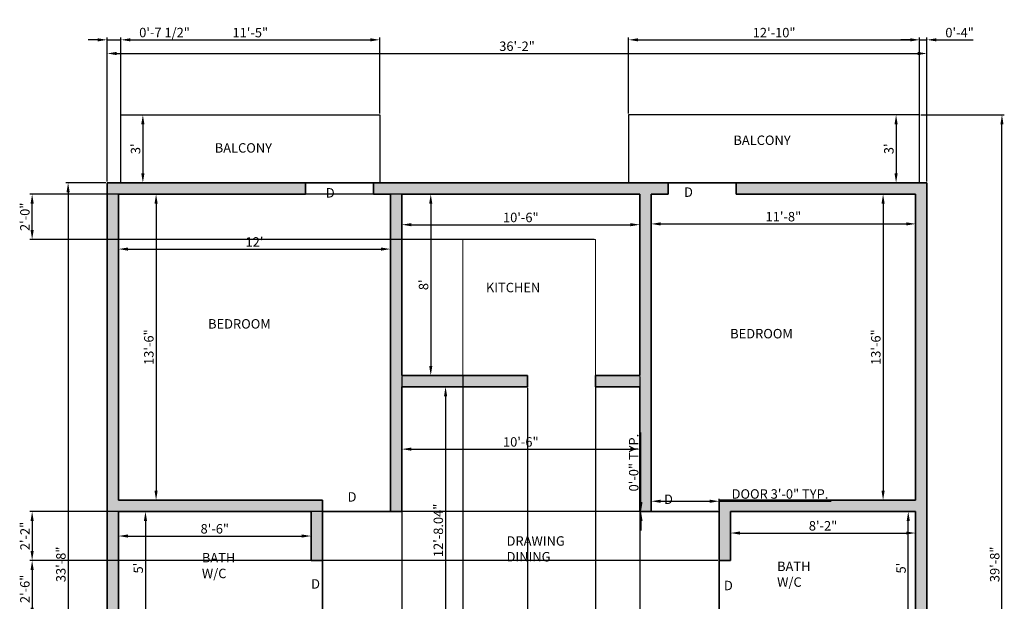
# Model space of a CAD drawing. Units: inches. Extents: x -48 to 476, y -487 to 101.
# Tile 2 of 2: x -48 to 473, y -207 to 101. Entities that reach past the tile are written whole.
import ezdxf

# ---------------------------------------------------------------- set-up
doc = ezdxf.new("R2010")
doc.units = ezdxf.units.IN
for name, color, linetype, lineweight in [('A-ANNO-DIMS', 2, 'Continuous', 18), ('A-ANNO-TEXT', 7, 'Continuous', 18), ('A-AREA-IDEN', 7, 'Continuous', 18), ('A-DOOR', 4, 'Continuous', 25), ('A-FLOR-BALC', 7, 'Continuous', 25), ('A-FLOR-FIXT', 8, 'Continuous', 18), ('A-WALL', 7, 'Continuous', 35), ('A-WALL-PATT', 1, 'Continuous', 13)]:
    doc.layers.add(name, color=color, linetype=linetype, lineweight=lineweight)
doc.styles.get("Standard").update_dxf_attribs({"font": 'arial.ttf'})
doc.dimstyles.new('ISO-25', dxfattribs={"dimtxt": 5, "dimasz": 5, "dimexe": 1.25, "dimexo": 0.625, "dimtad": 1, "dimlunit": 3, "dimtxsty": 'Standard', "dimcen": 2.5, "dimadec": 0, "dimazin": 0, "dimtfac": 1, "dimtmove": 0, "dimatfit": 3, "dimfxl": 1, "dimarcsym": 0})

# ---------------------------------------------------------------- blocks, each defined once
blk = doc.blocks.new('*D1')
at = {"layer": 'A-ANNO-DIMS', "color": 0, "lineweight": -2, "transparency": 16777216}
for p, q in [((4.01, -14.47), (4.01, -21.47)), ((148.01, -14.47), (148.01, -21.47)), ((9.01, -20.22), (143.01, -20.22))]:
    blk.add_line(p, q, dxfattribs=at)
at = {"layer": 'A-ANNO-DIMS', "color": 0, "transparency": 16777216}
for points in [[(9.01, -19.39), (9.01, -21.06), (4.01, -20.22)], [(143.01, -19.39), (143.01, -21.06), (148.01, -20.22)]]:
    blk.add_solid(points, dxfattribs=at)
at = {"layer": 'Defpoints', "color": 0, "transparency": 16777216}
for p in [(4.01, -13.85), (148.01, -13.85), (148.01, -20.22)]:
    blk.add_point(p, dxfattribs=at)
at = {"layer": 'A-ANNO-DIMS', "color": 0, "transparency": 16777216, "insert": (76.01, -17.09), "char_height": 5, "attachment_point": 5}
blk.add_mtext("12'", dxfattribs=at)
blk = doc.blocks.new('*D2')
at = {"layer": 'A-ANNO-DIMS', "color": 0, "lineweight": -2, "transparency": 16777216}
for p, q in [((4.64, 8.87), (25.17, 8.87)), ((23.92, 3.87), (23.92, -148.13)), ((4.64, -153.13), (25.17, -153.13))]:
    blk.add_line(p, q, dxfattribs=at)
at = {"layer": 'A-ANNO-DIMS', "color": 0, "transparency": 16777216}
for points in [[(23.09, 3.87), (24.75, 3.87), (23.92, 8.87)], [(23.09, -148.13), (24.75, -148.13), (23.92, -153.13)]]:
    blk.add_solid(points, dxfattribs=at)
at = {"layer": 'Defpoints', "color": 0, "transparency": 16777216}
for p in [(4.01, 8.87), (4.01, -153.13), (23.92, -153.13)]:
    blk.add_point(p, dxfattribs=at)
at = {"layer": 'A-ANNO-DIMS', "color": 0, "transparency": 16777216, "insert": (20.74, -72.13), "char_height": 5, "attachment_point": 5, "rotation": 90}
blk.add_mtext('13\'-6"', dxfattribs=at)
blk = doc.blocks.new('*D3')
at = {"layer": 'A-ANNO-DIMS', "color": 0, "lineweight": -2, "transparency": 16777216}
for p, q in [((154.01, 8.24), (154.01, -8.55)), ((280.01, 8.24), (280.01, -8.55)), ((159.01, -7.3), (275.01, -7.3))]:
    blk.add_line(p, q, dxfattribs=at)
at = {"layer": 'A-ANNO-DIMS', "color": 0, "transparency": 16777216}
for points in [[(159.01, -6.47), (159.01, -8.13), (154.01, -7.3)], [(275.01, -6.47), (275.01, -8.13), (280.01, -7.3)]]:
    blk.add_solid(points, dxfattribs=at)
at = {"layer": 'Defpoints', "color": 0, "transparency": 16777216}
for p in [(154.01, 8.87), (280.01, 8.87), (280.01, -7.3)]:
    blk.add_point(p, dxfattribs=at)
at = {"layer": 'A-ANNO-DIMS', "color": 0, "transparency": 16777216, "insert": (217.01, -4.12), "char_height": 5, "attachment_point": 5}
blk.add_mtext('10\'-6"', dxfattribs=at)
blk = doc.blocks.new('*D4')
at = {"layer": 'A-ANNO-DIMS', "color": 0, "lineweight": -2, "transparency": 16777216}
for p, q in [((154.64, 8.87), (170.59, 8.87)), ((169.34, 3.87), (169.34, -82.13)), ((154.64, -87.13), (170.59, -87.13))]:
    blk.add_line(p, q, dxfattribs=at)
at = {"layer": 'A-ANNO-DIMS', "color": 0, "transparency": 16777216}
for points in [[(168.51, 3.87), (170.17, 3.87), (169.34, 8.87)], [(168.51, -82.13), (170.17, -82.13), (169.34, -87.13)]]:
    blk.add_solid(points, dxfattribs=at)
at = {"layer": 'Defpoints', "color": 0, "transparency": 16777216}
for p in [(154.01, 8.87), (154.01, -87.13), (169.34, -87.13)]:
    blk.add_point(p, dxfattribs=at)
at = {"layer": 'A-ANNO-DIMS', "color": 0, "transparency": 16777216, "insert": (166.16, -39.13), "char_height": 5, "attachment_point": 5, "rotation": 90}
blk.add_mtext("8'", dxfattribs=at)
blk = doc.blocks.new('*D5')
at = {"layer": 'A-ANNO-DIMS', "color": 0, "lineweight": -2, "transparency": 16777216}
for p, q in [((154.01, -125.51), (154.01, -124.88)), ((280.01, -125.51), (280.01, -124.88)), ((159.01, -126.13), (275.01, -126.13))]:
    blk.add_line(p, q, dxfattribs=at)
at = {"layer": 'A-ANNO-DIMS', "color": 0, "transparency": 16777216}
for points in [[(159.01, -125.3), (159.01, -126.97), (154.01, -126.13)], [(275.01, -125.3), (275.01, -126.97), (280.01, -126.13)]]:
    blk.add_solid(points, dxfattribs=at)
at = {"layer": 'Defpoints', "color": 0, "transparency": 16777216}
for p in [(154.01, -126.13), (280.01, -126.13), (280.01, -126.13)]:
    blk.add_point(p, dxfattribs=at)
at = {"layer": 'A-ANNO-DIMS', "color": 0, "transparency": 16777216, "insert": (217.01, -122.96), "char_height": 5, "attachment_point": 5}
blk.add_mtext('10\'-6"', dxfattribs=at)
blk = doc.blocks.new('*D6')
at = {"layer": 'A-ANNO-DIMS', "color": 0, "lineweight": -2, "transparency": 16777216}
for p, q in [((286.01, -2.3), (286.01, -8.13)), ((426.01, -2.3), (426.01, -8.13)), ((291.01, -6.88), (421.01, -6.88))]:
    blk.add_line(p, q, dxfattribs=at)
at = {"layer": 'A-ANNO-DIMS', "color": 0, "transparency": 16777216}
for points in [[(291.01, -6.05), (291.01, -7.72), (286.01, -6.88)], [(421.01, -6.05), (421.01, -7.72), (426.01, -6.88)]]:
    blk.add_solid(points, dxfattribs=at)
at = {"layer": 'Defpoints', "color": 0, "transparency": 16777216}
for p in [(286.01, -1.67), (426.01, -1.67), (426.01, -6.88)]:
    blk.add_point(p, dxfattribs=at)
at = {"layer": 'A-ANNO-DIMS', "color": 0, "transparency": 16777216, "insert": (356.01, -3.7), "char_height": 5, "attachment_point": 5}
blk.add_mtext('11\'-8"', dxfattribs=at)
blk = doc.blocks.new('*D7')
at = {"layer": 'A-ANNO-DIMS', "color": 0, "lineweight": -2, "transparency": 16777216}
for p, q in [((425.39, 8.87), (407.53, 8.87)), ((408.78, 3.87), (408.78, -148.13)), ((425.39, -153.13), (407.53, -153.13))]:
    blk.add_line(p, q, dxfattribs=at)
at = {"layer": 'A-ANNO-DIMS', "color": 0, "transparency": 16777216}
for points in [[(407.95, 3.87), (409.62, 3.87), (408.78, 8.87)], [(407.95, -148.13), (409.62, -148.13), (408.78, -153.13)]]:
    blk.add_solid(points, dxfattribs=at)
at = {"layer": 'Defpoints', "color": 0, "transparency": 16777216}
for p in [(426.01, 8.87), (408.78, -153.13), (426.01, -153.13)]:
    blk.add_point(p, dxfattribs=at)
at = {"layer": 'A-ANNO-DIMS', "color": 0, "transparency": 16777216, "insert": (405.6, -72.13), "char_height": 5, "attachment_point": 5, "rotation": 90}
blk.add_mtext('13\'-6"', dxfattribs=at)
blk = doc.blocks.new('*D8')
at = {"layer": 'A-ANNO-DIMS', "color": 0, "lineweight": -2, "transparency": 16777216}
for p, q in [((328.01, -159.76), (328.01, -171.8)), ((426.01, -159.76), (426.01, -171.8)), ((333.01, -170.55), (421.01, -170.55))]:
    blk.add_line(p, q, dxfattribs=at)
at = {"layer": 'A-ANNO-DIMS', "color": 0, "transparency": 16777216}
for points in [[(333.01, -169.72), (333.01, -171.38), (328.01, -170.55)], [(421.01, -169.72), (421.01, -171.38), (426.01, -170.55)]]:
    blk.add_solid(points, dxfattribs=at)
at = {"layer": 'Defpoints', "color": 0, "transparency": 16777216}
for p in [(328.01, -159.13), (426.01, -159.13), (426.01, -170.55)]:
    blk.add_point(p, dxfattribs=at)
at = {"layer": 'A-ANNO-DIMS', "color": 0, "transparency": 16777216, "insert": (377.01, -167.37), "char_height": 5, "attachment_point": 5}
blk.add_mtext('8\'-2"', dxfattribs=at)
blk = doc.blocks.new('*D9')
at = {"layer": 'A-ANNO-DIMS', "color": 0, "lineweight": -2, "transparency": 16777216}
for p, q in [((425.39, -159.13), (420.87, -159.13)), ((422.12, -214.13), (422.12, -164.13)), ((425.39, -219.13), (420.87, -219.13))]:
    blk.add_line(p, q, dxfattribs=at)
at = {"layer": 'A-ANNO-DIMS', "color": 0, "transparency": 16777216}
for points in [[(421.29, -164.13), (422.95, -164.13), (422.12, -159.13)], [(421.29, -214.13), (422.95, -214.13), (422.12, -219.13)]]:
    blk.add_solid(points, dxfattribs=at)
at = {"layer": 'Defpoints', "color": 0, "transparency": 16777216}
for p in [(422.12, -159.13), (426.01, -159.13), (426.01, -219.13)]:
    blk.add_point(p, dxfattribs=at)
at = {"layer": 'A-ANNO-DIMS', "color": 0, "transparency": 16777216, "insert": (418.95, -189.13), "char_height": 5, "attachment_point": 5, "rotation": 90}
blk.add_mtext("5'", dxfattribs=at)
blk = doc.blocks.new('*D20')
at = {"layer": 'A-ANNO-DIMS', "color": 0, "lineweight": -2, "transparency": 16777216}
for p, q in [((4.01, -159.76), (4.01, -173.38)), ((106.01, -159.76), (106.01, -173.38)), ((9.01, -172.13), (101.01, -172.13))]:
    blk.add_line(p, q, dxfattribs=at)
at = {"layer": 'A-ANNO-DIMS', "color": 0, "transparency": 16777216}
for points in [[(9.01, -171.3), (9.01, -172.97), (4.01, -172.13)], [(101.01, -171.3), (101.01, -172.97), (106.01, -172.13)]]:
    blk.add_solid(points, dxfattribs=at)
at = {"layer": 'Defpoints', "color": 0, "transparency": 16777216}
for p in [(4.01, -159.13), (106.01, -159.13), (106.01, -172.13)]:
    blk.add_point(p, dxfattribs=at)
at = {"layer": 'A-ANNO-DIMS', "color": 0, "transparency": 16777216, "insert": (55.01, -168.96), "char_height": 5, "attachment_point": 5}
blk.add_mtext('8\'-6"', dxfattribs=at)
blk = doc.blocks.new('*D21')
at = {"layer": 'A-ANNO-DIMS', "color": 0, "lineweight": -2, "transparency": 16777216}
for p, q in [((4.64, -159.13), (19.56, -159.13)), ((18.31, -164.13), (18.31, -214.13)), ((4.64, -219.13), (19.56, -219.13))]:
    blk.add_line(p, q, dxfattribs=at)
at = {"layer": 'A-ANNO-DIMS', "color": 0, "transparency": 16777216}
for points in [[(17.48, -164.13), (19.15, -164.13), (18.31, -159.13)], [(17.48, -214.13), (19.15, -214.13), (18.31, -219.13)]]:
    blk.add_solid(points, dxfattribs=at)
at = {"layer": 'Defpoints', "color": 0, "transparency": 16777216}
for p in [(4.01, -159.13), (4.01, -219.13), (18.31, -219.13)]:
    blk.add_point(p, dxfattribs=at)
at = {"layer": 'A-ANNO-DIMS', "color": 0, "transparency": 16777216, "insert": (15.14, -189.13), "char_height": 5, "attachment_point": 5, "rotation": 90}
blk.add_mtext("5'", dxfattribs=at)
blk = doc.blocks.new('*D22')
at = {"layer": 'A-ANNO-DIMS', "color": 0, "lineweight": -2, "transparency": 16777216}
for p, q in [((154.64, -93.13), (178.42, -93.13)), ((177.17, -98.13), (177.17, -240.18)), ((154.64, -245.18), (178.42, -245.18))]:
    blk.add_line(p, q, dxfattribs=at)
at = {"layer": 'A-ANNO-DIMS', "color": 0, "transparency": 16777216}
for points in [[(176.34, -98.13), (178, -98.13), (177.17, -93.13)], [(176.34, -240.18), (178, -240.18), (177.17, -245.18)]]:
    blk.add_solid(points, dxfattribs=at)
at = {"layer": 'Defpoints', "color": 0, "transparency": 16777216}
for p in [(154.01, -93.13), (154.01, -245.18), (177.17, -245.18)]:
    blk.add_point(p, dxfattribs=at)
at = {"layer": 'A-ANNO-DIMS', "color": 0, "transparency": 16777216, "insert": (173.99, -169.15), "char_height": 5, "attachment_point": 5, "rotation": 90}
blk.add_mtext('12\'-8.04"', dxfattribs=at)
blk = doc.blocks.new('*D23')
at = {"layer": 'A-ANNO-DIMS', "color": 0, "lineweight": -2, "transparency": 16777216}
for p, q in [((5.93, 50.87), (18.17, 50.87)), ((16.92, 45.87), (16.92, 19.87)), ((5.93, 14.87), (18.17, 14.87))]:
    blk.add_line(p, q, dxfattribs=at)
at = {"layer": 'A-ANNO-DIMS', "color": 0, "transparency": 16777216}
for points in [[(16.08, 45.87), (17.75, 45.87), (16.92, 50.87)], [(16.08, 19.87), (17.75, 19.87), (16.92, 14.87)]]:
    blk.add_solid(points, dxfattribs=at)
at = {"layer": 'Defpoints', "color": 0, "transparency": 16777216}
for p in [(5.3, 50.87), (5.3, 14.87), (16.92, 14.87)]:
    blk.add_point(p, dxfattribs=at)
at = {"layer": 'A-ANNO-DIMS', "color": 0, "transparency": 16777216, "insert": (13.74, 32.87), "char_height": 5, "attachment_point": 5, "rotation": 90}
blk.add_mtext("3'", dxfattribs=at)
blk = doc.blocks.new('*D24')
at = {"layer": 'A-ANNO-DIMS', "color": 0, "lineweight": -2, "transparency": 16777216}
for p, q in [((427.52, 50.87), (414.43, 50.87)), ((415.68, 45.87), (415.68, 19.87)), ((427.52, 14.87), (414.43, 14.87))]:
    blk.add_line(p, q, dxfattribs=at)
at = {"layer": 'A-ANNO-DIMS', "color": 0, "transparency": 16777216}
for points in [[(414.84, 45.87), (416.51, 45.87), (415.68, 50.87)], [(414.84, 19.87), (416.51, 19.87), (415.68, 14.87)]]:
    blk.add_solid(points, dxfattribs=at)
at = {"layer": 'Defpoints', "color": 0, "transparency": 16777216}
for p in [(428.14, 50.87), (415.68, 14.87), (428.14, 14.87)]:
    blk.add_point(p, dxfattribs=at)
at = {"layer": 'A-ANNO-DIMS', "color": 0, "transparency": 16777216, "insert": (412.5, 32.87), "char_height": 5, "attachment_point": 5, "rotation": 90}
blk.add_mtext("3'", dxfattribs=at)
blk = doc.blocks.new('*D25')
at = {"layer": 'A-ANNO-DIMS', "color": 0, "lineweight": -2, "transparency": 16777216}
for p, q in [((-1.99, 15.49), (-1.99, 84.59)), ((432.01, 15.49), (432.01, 84.59)), ((3.01, 83.34), (427.01, 83.34))]:
    blk.add_line(p, q, dxfattribs=at)
at = {"layer": 'A-ANNO-DIMS', "color": 0, "transparency": 16777216}
for points in [[(3.01, 84.17), (3.01, 82.5), (-1.99, 83.34)], [(427.01, 84.17), (427.01, 82.5), (432.01, 83.34)]]:
    blk.add_solid(points, dxfattribs=at)
at = {"layer": 'Defpoints', "color": 0, "transparency": 16777216}
for p in [(432.01, 83.34), (-1.99, 14.87), (432.01, 14.87)]:
    blk.add_point(p, dxfattribs=at)
at = {"layer": 'A-ANNO-DIMS', "color": 0, "transparency": 16777216, "insert": (215.01, 86.52), "char_height": 5, "attachment_point": 5}
blk.add_mtext('36\'-2"', dxfattribs=at)
blk = doc.blocks.new('*D26')
at = {"layer": 'A-ANNO-DIMS', "color": 0, "lineweight": -2, "transparency": 16777216}
for p, q in [((-2.61, 14.87), (-23.89, 14.87)), ((-22.64, 9.87), (-22.64, -384.13)), ((-2.61, -389.13), (-23.89, -389.13))]:
    blk.add_line(p, q, dxfattribs=at)
at = {"layer": 'A-ANNO-DIMS', "color": 0, "transparency": 16777216}
for points in [[(-23.48, 9.87), (-21.81, 9.87), (-22.64, 14.87)], [(-23.48, -384.13), (-21.81, -384.13), (-22.64, -389.13)]]:
    blk.add_solid(points, dxfattribs=at)
at = {"layer": 'Defpoints', "color": 0, "transparency": 16777216}
for p in [(-1.99, 14.87), (-22.64, -389.13), (-1.99, -389.13)]:
    blk.add_point(p, dxfattribs=at)
at = {"layer": 'A-ANNO-DIMS', "color": 0, "transparency": 16777216, "insert": (-25.82, -187.13), "char_height": 5, "attachment_point": 5, "rotation": 90}
blk.add_mtext('33\'-8"', dxfattribs=at)
blk = doc.blocks.new('DOOR-36-CLOSED')
blk.add_line((0, 0), (36, 0))
blk = doc.blocks.new('*D29')
at = {"layer": 'A-ANNO-DIMS', "color": 0, "lineweight": -2, "transparency": 16777216}
for p, q in [((286.01, -158.51), (286.01, -152.48)), ((291.01, -153.73), (317.01, -153.73)), ((322.01, -158.51), (322.01, -152.48)), ((322.01, -153.73), (381.38, -153.73))]:
    blk.add_line(p, q, dxfattribs=at)
at = {"layer": 'A-ANNO-DIMS', "color": 0, "transparency": 16777216}
for points in [[(291.01, -152.9), (291.01, -154.57), (286.01, -153.73)], [(317.01, -152.9), (317.01, -154.57), (322.01, -153.73)]]:
    blk.add_solid(points, dxfattribs=at)
at = {"layer": 'Defpoints', "color": 0, "transparency": 16777216}
for p in [(322.01, -153.73), (286.01, -159.13), (322.01, -159.13)]:
    blk.add_point(p, dxfattribs=at)
at = {"layer": 'A-ANNO-DIMS', "color": 0, "transparency": 16777216, "insert": (354.2, -150.52), "char_height": 5, "attachment_point": 5}
blk.add_mtext('DOOR 3\'-0" TYP.', dxfattribs=at)
blk = doc.blocks.new('*D30')
at = {"layer": 'A-ANNO-DIMS', "color": 0, "lineweight": -2, "transparency": 16777216}
for p, q in [((280.61, -154.13), (280.61, -117.41)), ((285.39, -159.13), (279.36, -159.13)), ((285.39, -159.13), (279.36, -159.13)), ((280.61, -164.13), (280.61, -169.13))]:
    blk.add_line(p, q, dxfattribs=at)
at = {"layer": 'A-ANNO-DIMS', "color": 0, "transparency": 16777216}
for points in [[(279.78, -154.13), (281.44, -154.13), (280.61, -159.13)], [(279.78, -164.13), (281.44, -164.13), (280.61, -159.13)]]:
    blk.add_solid(points, dxfattribs=at)
at = {"layer": 'Defpoints', "color": 0, "transparency": 16777216}
for p in [(280.61, -159.13), (286.01, -159.13), (286.01, -159.13)]:
    blk.add_point(p, dxfattribs=at)
at = {"layer": 'A-ANNO-DIMS', "color": 0, "transparency": 16777216, "insert": (277.43, -133.27), "char_height": 5, "attachment_point": 5, "rotation": 90}
blk.add_mtext('0\'-0" TYP.', dxfattribs=at)
blk = doc.blocks.new('*D33')
at = {"layer": 'A-ANNO-DIMS', "color": 0, "lineweight": -2, "transparency": 16777216}
for p, q in [((428.77, 50.87), (472.96, 50.87)), ((471.71, -420.13), (471.71, 45.87)), ((428.76, -425.13), (472.96, -425.13))]:
    blk.add_line(p, q, dxfattribs=at)
at = {"layer": 'A-ANNO-DIMS', "color": 0, "transparency": 16777216}
for points in [[(470.88, 45.87), (472.54, 45.87), (471.71, 50.87)], [(470.88, -420.13), (472.54, -420.13), (471.71, -425.13)]]:
    blk.add_solid(points, dxfattribs=at)
at = {"layer": 'Defpoints', "color": 0, "transparency": 16777216}
for p in [(428.14, 50.87), (471.71, 50.87), (428.14, -425.13)]:
    blk.add_point(p, dxfattribs=at)
at = {"layer": 'A-ANNO-DIMS', "color": 0, "transparency": 16777216, "insert": (468.53, -187.13), "char_height": 5, "attachment_point": 5, "rotation": 90}
blk.add_mtext('39\'-8"', dxfattribs=at)
blk = doc.blocks.new('*D34')
at = {"layer": 'A-ANNO-DIMS', "color": 0, "lineweight": -2, "transparency": 16777216}
for p, q in [((5.3, 51.49), (5.3, 91.82)), ((10.3, 90.57), (137.3, 90.57)), ((142.3, 51.49), (142.3, 91.82))]:
    blk.add_line(p, q, dxfattribs=at)
at = {"layer": 'A-ANNO-DIMS', "color": 0, "transparency": 16777216}
for points in [[(10.3, 91.4), (10.3, 89.73), (5.3, 90.57)], [(137.3, 91.4), (137.3, 89.73), (142.3, 90.57)]]:
    blk.add_solid(points, dxfattribs=at)
at = {"layer": 'Defpoints', "color": 0, "transparency": 16777216}
for p in [(142.3, 90.57), (5.3, 50.87), (142.3, 50.87)]:
    blk.add_point(p, dxfattribs=at)
at = {"layer": 'A-ANNO-DIMS', "color": 0, "transparency": 16777216, "insert": (73.8, 93.74), "char_height": 5, "attachment_point": 5}
blk.add_mtext('11\'-5"', dxfattribs=at)
blk = doc.blocks.new('*D35')
at = {"layer": 'A-ANNO-DIMS', "color": 0, "lineweight": -2, "transparency": 16777216}
for p, q in [((274.06, 51.49), (274.06, 91.82)), ((279.06, 90.57), (423.14, 90.57)), ((428.14, 51.49), (428.14, 91.82))]:
    blk.add_line(p, q, dxfattribs=at)
at = {"layer": 'A-ANNO-DIMS', "color": 0, "transparency": 16777216}
for points in [[(279.06, 91.4), (279.06, 89.73), (274.06, 90.57)], [(423.14, 91.4), (423.14, 89.73), (428.14, 90.57)]]:
    blk.add_solid(points, dxfattribs=at)
at = {"layer": 'Defpoints', "color": 0, "transparency": 16777216}
for p in [(428.14, 90.57), (274.06, 50.87), (428.14, 50.87)]:
    blk.add_point(p, dxfattribs=at)
at = {"layer": 'A-ANNO-DIMS', "color": 0, "transparency": 16777216, "insert": (351.1, 93.74), "char_height": 5, "attachment_point": 5}
blk.add_mtext('12\'-10"', dxfattribs=at)
blk = doc.blocks.new('*D36')
at = {"layer": 'A-ANNO-DIMS', "color": 0, "lineweight": -2, "transparency": 16777216}
for p, q in [((154.01, -87.76), (154.01, -466.08)), ((186.37, -87.76), (186.37, -466.08)), ((159.01, -464.83), (181.37, -464.83))]:
    blk.add_line(p, q, dxfattribs=at)
at = {"layer": 'A-ANNO-DIMS', "color": 0, "transparency": 16777216}
for points in [[(159.01, -464), (159.01, -465.67), (154.01, -464.83)], [(181.37, -464), (181.37, -465.67), (186.37, -464.83)]]:
    blk.add_solid(points, dxfattribs=at)
at = {"layer": 'Defpoints', "color": 0, "transparency": 16777216}
for p in [(154.01, -87.13), (186.37, -87.13), (186.37, -464.83)]:
    blk.add_point(p, dxfattribs=at)
at = {"layer": 'A-ANNO-DIMS', "color": 0, "transparency": 16777216, "insert": (170.19, -461.62), "char_height": 5, "attachment_point": 5}
blk.add_mtext('2\'-8 1/2"', dxfattribs=at)
blk = doc.blocks.new('*D37')
at = {"layer": 'A-ANNO-DIMS', "color": 0, "lineweight": -2, "transparency": 16777216}
for p, q in [((256.47, -87.76), (256.47, -466.08)), ((280.01, -87.76), (280.01, -466.08)), ((261.47, -464.83), (275.01, -464.83)), ((280.01, -464.83), (314.62, -464.83))]:
    blk.add_line(p, q, dxfattribs=at)
at = {"layer": 'A-ANNO-DIMS', "color": 0, "transparency": 16777216}
for points in [[(261.47, -464), (261.47, -465.67), (256.47, -464.83)], [(275.01, -464), (275.01, -465.67), (280.01, -464.83)]]:
    blk.add_solid(points, dxfattribs=at)
at = {"layer": 'Defpoints', "color": 0, "transparency": 16777216}
for p in [(256.47, -87.13), (280.01, -87.13), (280.01, -464.83)]:
    blk.add_point(p, dxfattribs=at)
at = {"layer": 'A-ANNO-DIMS', "color": 0, "transparency": 16777216, "insert": (299.81, -461.62), "char_height": 5, "attachment_point": 5}
blk.add_mtext('1\'-11 1/2"', dxfattribs=at)
blk = doc.blocks.new('*D38')
at = {"layer": 'A-ANNO-DIMS', "color": 0, "lineweight": -2, "transparency": 16777216}
for p, q in [((279.39, 8.87), (-42.94, 8.87)), ((-41.69, -10.13), (-41.69, 3.87)), ((255.85, -15.13), (-42.94, -15.13))]:
    blk.add_line(p, q, dxfattribs=at)
at = {"layer": 'A-ANNO-DIMS', "color": 0, "transparency": 16777216}
for points in [[(-42.52, 3.87), (-40.86, 3.87), (-41.69, 8.87)], [(-42.52, -10.13), (-40.86, -10.13), (-41.69, -15.13)]]:
    blk.add_solid(points, dxfattribs=at)
at = {"layer": 'Defpoints', "color": 0, "transparency": 16777216}
for p in [(-41.69, 8.87), (280.01, 8.87), (256.47, -15.13)]:
    blk.add_point(p, dxfattribs=at)
at = {"layer": 'A-ANNO-DIMS', "color": 0, "transparency": 16777216, "insert": (-44.87, -3.13), "char_height": 5, "attachment_point": 5, "rotation": 90}
blk.add_mtext('2\'-0"', dxfattribs=at)
blk = doc.blocks.new('*D39')
at = {"layer": 'A-ANNO-DIMS', "color": 0, "lineweight": -2, "transparency": 16777216}
for p, q in [((220.47, -93.76), (220.47, -466.08)), ((256.47, -93.76), (256.47, -466.08)), ((225.47, -464.83), (251.47, -464.83))]:
    blk.add_line(p, q, dxfattribs=at)
at = {"layer": 'A-ANNO-DIMS', "color": 0, "transparency": 16777216}
for points in [[(225.47, -464), (225.47, -465.67), (220.47, -464.83)], [(251.47, -464), (251.47, -465.67), (256.47, -464.83)]]:
    blk.add_solid(points, dxfattribs=at)
at = {"layer": 'Defpoints', "color": 0, "transparency": 16777216}
for p in [(220.47, -93.13), (256.47, -93.13), (256.47, -464.83)]:
    blk.add_point(p, dxfattribs=at)
at = {"layer": 'A-ANNO-DIMS', "color": 0, "transparency": 16777216, "insert": (238.47, -461.65), "char_height": 5, "attachment_point": 5}
blk.add_mtext('3\'-0"', dxfattribs=at)
blk = doc.blocks.new('*D41')
at = {"layer": 'A-ANNO-DIMS', "color": 0, "lineweight": -2, "transparency": 16777216}
for p, q in [((321.39, -159.13), (-42.94, -159.13)), ((-41.69, -164.13), (-41.69, -180.13)), ((321.39, -185.13), (-42.94, -185.13))]:
    blk.add_line(p, q, dxfattribs=at)
at = {"layer": 'A-ANNO-DIMS', "color": 0, "transparency": 16777216}
for points in [[(-42.52, -164.13), (-40.86, -164.13), (-41.69, -159.13)], [(-42.52, -180.13), (-40.86, -180.13), (-41.69, -185.13)]]:
    blk.add_solid(points, dxfattribs=at)
at = {"layer": 'Defpoints', "color": 0, "transparency": 16777216}
for p in [(322.01, -159.13), (-41.69, -185.13), (322.01, -185.13)]:
    blk.add_point(p, dxfattribs=at)
at = {"layer": 'A-ANNO-DIMS', "color": 0, "transparency": 16777216, "insert": (-44.82, -172.13), "char_height": 5, "attachment_point": 5, "rotation": 90}
blk.add_mtext('2\'-2"', dxfattribs=at)
blk = doc.blocks.new('*D42')
at = {"layer": 'A-ANNO-DIMS', "color": 0, "lineweight": -2, "transparency": 16777216}
for p, q in [((321.39, -185.13), (-42.94, -185.13)), ((-41.69, -190.13), (-41.69, -210.13)), ((321.39, -215.13), (-42.94, -215.13))]:
    blk.add_line(p, q, dxfattribs=at)
at = {"layer": 'A-ANNO-DIMS', "color": 0, "transparency": 16777216}
for points in [[(-42.52, -190.13), (-40.86, -190.13), (-41.69, -185.13)], [(-42.52, -210.13), (-40.86, -210.13), (-41.69, -215.13)]]:
    blk.add_solid(points, dxfattribs=at)
at = {"layer": 'Defpoints', "color": 0, "transparency": 16777216}
for p in [(322.01, -185.13), (-41.69, -215.13), (322.01, -215.13)]:
    blk.add_point(p, dxfattribs=at)
at = {"layer": 'A-ANNO-DIMS', "color": 0, "transparency": 16777216, "insert": (-44.87, -200.13), "char_height": 5, "attachment_point": 5, "rotation": 90}
blk.add_mtext('2\'-6"', dxfattribs=at)
blk = doc.blocks.new('*D46')
at = {"layer": 'A-ANNO-DIMS', "color": 0, "lineweight": -2, "transparency": 16777216}
for p, q in [((-6.99, 90.57), (-11.99, 90.57)), ((-1.99, 15.49), (-1.99, 91.82)), ((-1.99, 90.57), (5.3, 90.57)), ((5.3, 15.49), (5.3, 91.82)), ((10.3, 90.57), (41.49, 90.57))]:
    blk.add_line(p, q, dxfattribs=at)
at = {"layer": 'A-ANNO-DIMS', "color": 0, "transparency": 16777216}
for points in [[(-6.99, 91.4), (-6.99, 89.73), (-1.99, 90.57)], [(10.3, 91.4), (10.3, 89.73), (5.3, 90.57)]]:
    blk.add_solid(points, dxfattribs=at)
at = {"layer": 'Defpoints', "color": 0, "transparency": 16777216}
for p in [(5.3, 90.57), (-1.99, 14.87), (5.3, 14.87)]:
    blk.add_point(p, dxfattribs=at)
at = {"layer": 'A-ANNO-DIMS', "color": 0, "transparency": 16777216, "insert": (28.4, 93.78), "char_height": 5, "attachment_point": 5}
blk.add_mtext('0\'-7 1/2"', dxfattribs=at)
blk = doc.blocks.new('*D47')
at = {"layer": 'A-ANNO-DIMS', "color": 0, "lineweight": -2, "transparency": 16777216}
for p, q in [((423.14, 90.57), (418.14, 90.57)), ((428.14, 15.49), (428.14, 91.82)), ((428.14, 90.57), (432.01, 90.57)), ((432.01, 15.49), (432.01, 91.82)), ((437.01, 90.57), (456.55, 90.57))]:
    blk.add_line(p, q, dxfattribs=at)
at = {"layer": 'A-ANNO-DIMS', "color": 0, "transparency": 16777216}
for points in [[(423.14, 91.4), (423.14, 89.73), (428.14, 90.57)], [(437.01, 91.4), (437.01, 89.73), (432.01, 90.57)]]:
    blk.add_solid(points, dxfattribs=at)
at = {"layer": 'Defpoints', "color": 0, "transparency": 16777216}
for p in [(432.01, 90.57), (428.14, 14.87), (432.01, 14.87)]:
    blk.add_point(p, dxfattribs=at)
at = {"layer": 'A-ANNO-DIMS', "color": 0, "transparency": 16777216, "insert": (449.28, 93.74), "char_height": 5, "attachment_point": 5}
blk.add_mtext('0\'-4"', dxfattribs=at)

msp = doc.modelspace()

# ---------------------------------------------------------------- hatches: boundary and pattern name
at = {"layer": 'A-WALL-PATT'}
h = msp.add_hatch(color=256, dxfattribs=at)
h.dxf.hatch_style = 1
h.paths.add_polyline_path([(103.011, 14.867), (-1.989, 14.867), (-1.989, -389.133), (103.011, -389.133), (103.011, -383.133), (4.011, -383.133), (4.011, -225.133), (112.011, -225.133), (112.011, -215.133), (106.011, -215.133), (106.011, -219.133), (4.011, -219.133), (4.011, -159.133), (106.011, -159.133), (106.011, -185.133), (112.011, -185.133), (112.011, -159.133), (112.011, -153.133), (4.011, -153.133), (4.011, 8.867), (103.011, 8.867)])
h.paths.add_polyline_path([(295.011, 14.867), (139.011, 14.867), (139.011, 8.867), (148.011, 8.867), (148.011, -159.133), (154.011, -159.133), (154.011, -93.133), (220.474, -93.133), (220.474, -87.133), (154.011, -87.133), (154.011, 8.867), (280.011, 8.867), (280.011, -87.133), (256.474, -87.133), (256.474, -93.133), (280.011, -93.133), (280.011, -159.133), (286.011, -159.133), (286.011, 8.867), (295.011, 8.867)])
h.paths.add_polyline_path([(432.011, 14.867), (331.011, 14.867), (331.011, 8.867), (426.011, 8.867), (426.011, -153.133), (322.011, -153.133), (322.011, -159.133), (322.011, -185.133), (328.011, -185.133), (328.011, -159.133), (426.011, -159.133), (426.011, -219.133), (328.011, -219.133), (328.011, -215.133), (322.011, -215.133), (322.011, -225.133), (426.011, -225.133), (426.011, -383.133), (331.011, -383.133), (331.011, -389.133), (432.011, -389.133)])
h.paths.add_polyline_path([(295.011, -383.133), (286.011, -383.133), (286.011, -219.133), (280.011, -219.133), (280.011, -389.133), (289.971, -389.133), (295.011, -389.133)])
h.paths.add_polyline_path([(231.632, -245.175), (225.632, -245.175), (225.632, -383.133), (154.011, -383.133), (154.011, -219.133), (148.011, -219.133), (148.011, -383.133), (139.011, -383.133), (139.011, -389.133), (231.632, -389.133)])

# ---------------------------------------------------------------- linework, layer by layer
at = {"layer": 'A-FLOR-BALC'}
for p, q in [((5.301, 14.867), (5.301, 50.867)), ((5.301, 50.867), (142.295, 50.867)), ((142.295, 50.867), (142.295, 14.867)), ((428.141, 50.867), (274.056, 50.867)), ((274.056, 50.867), (274.056, 14.867)), ((428.141, 14.867), (428.141, 50.867))]:
    msp.add_line(p, q, dxfattribs=at)
at = {"layer": 'A-FLOR-FIXT'}
for p, q in [((186.373, -87.133), (186.373, -15.133)), ((186.373, -15.133), (256.474, -15.133)), ((256.474, -87.133), (256.474, -15.133))]:
    msp.add_line(p, q, dxfattribs=at)
at = {"layer": 'A-WALL'}
for p, q in [((-1.989, 14.867), (432.011, 14.867)), ((-1.989, -389.133), (-1.989, 14.867)), ((103.011, 8.867), (103.011, 14.867)), ((139.011, 8.867), (139.011, 14.867)), ((295.011, 8.867), (295.011, 14.867)), ((331.011, 8.867), (331.011, 14.867)), ((432.011, 14.867), (432.011, -389.133)), ((4.011, 8.867), (103.011, 8.867)), ((4.011, -153.133), (4.011, 8.867)), ((139.011, 8.867), (148.011, 8.867)), ((148.011, -159.133), (148.011, 8.867)), ((154.011, 8.867), (280.011, 8.867)), ((154.011, -87.133), (154.011, 8.867)), ((280.011, -87.133), (280.011, 8.867)), ((286.011, 8.867), (295.011, 8.867)), ((286.011, -159.133), (286.011, 8.867)), ((331.011, 8.867), (426.011, 8.867)), ((426.011, 8.867), (426.011, -153.133)), ((154.011, -87.133), (220.474, -87.133)), ((220.474, -87.133), (220.474, -93.133)), ((256.474, -87.133), (256.474, -93.133)), ((256.474, -87.133), (280.011, -87.133)), ((154.011, -93.133), (220.474, -93.133)), ((154.011, -159.133), (154.011, -93.133)), ((256.474, -93.133), (280.011, -93.133)), ((280.011, -159.133), (280.011, -93.133)), ((4.011, -153.133), (112.011, -153.133)), ((112.011, -153.133), (112.011, -159.133)), ((322.011, -153.133), (426.011, -153.133)), ((322.011, -153.133), (322.011, -159.133)), ((4.011, -159.133), (106.011, -159.133)), ((4.011, -219.133), (4.011, -159.133)), ((106.011, -159.133), (106.011, -185.133)), ((112.011, -159.133), (112.011, -225.133)), ((148.011, -159.133), (154.011, -159.133)), ((286.011, -159.133), (280.011, -159.133)), ((322.011, -159.133), (322.011, -225.133)), ((328.011, -159.133), (328.011, -185.133)), ((328.011, -159.133), (426.011, -159.133)), ((426.011, -159.133), (426.011, -219.133)), ((106.011, -185.133), (112.011, -185.133)), ((328.011, -185.133), (322.011, -185.133))]:
    msp.add_line(p, q, dxfattribs=at)

# ---------------------------------------------------------------- block references
at = {"layer": 'A-DOOR'}
for p in [(112.011, -159.133), (286.011, -159.133)]:
    msp.add_blockref('DOOR-36-CLOSED', p, dxfattribs=at)

# ---------------------------------------------------------------- texts
at = {"layer": 'A-ANNO-TEXT', "char_height": 5, "attachment_point": 1}
for width, insert in [(12.02496, (113.777, 12.087)), (15.21676, (303.425, 12.439)), (13.65541, (125.314, -148.923)), (12.90738, (292.835, -150.175)), (6, (106.011, -194.991)), (4.57283, (324.551, -195.821))]:
    msp.add_mtext_dynamic_manual_height_columns('D', width=width, gutter_width=12.5, heights=[0], dxfattribs=dict(at, insert=insert))
at = {"layer": 'A-AREA-IDEN', "char_height": 5, "attachment_point": 1}
for s, width, insert in [('BALCONY', 66.07909, (329.556, 39.904)), ('BALCONY', 79.83463, (54.985, 35.854)), ('KITCHEN', 49.61111, (198.547, -38.081)), ('BEDROOM', 51.87484, (51.455, -57.306)), ('BEDROOM', 70.87805, (327.852, -62.495)), ('DRAWING\\PDINING', 47.48367, (209.484, -172.264)), ('BATH\\PW/C', 59.46473, (48.174, -181.115)), ('BATH\\PW/C', 44.18732, (352.683, -185.687))]:
    msp.add_mtext_dynamic_manual_height_columns(s, width=width, gutter_width=12.5, heights=[0], dxfattribs=dict(at, insert=insert))

# ---------------------------------------------------------------- dimensions: what is measured, and where the dimension line sits
at = {"layer": 'A-ANNO-DIMS'}
for base, p1, p2, override, picture, middle in [((5.301, 90.567), (-1.989, 14.867), (5.301, 14.867), {"dimdec": 1, "dimlfac": 1, "dimrnd": 0, "dimzin": 1, "dimdsep": 46, "dimlunit": 4, "dimfrac": 2}, '*D46', (28.397, 93.777)), ((142.295, 90.567), (5.301, 50.867), (142.295, 50.867), {"dimdec": 1, "dimlfac": 1, "dimrnd": 0, "dimzin": 1, "dimdsep": 46, "dimlunit": 4, "dimfrac": 2}, '*D34', (73.798, 93.745)), ((428.141, 90.567), (274.056, 50.867), (428.141, 50.867), {"dimdec": 1, "dimlfac": 1, "dimrnd": 0, "dimzin": 1, "dimdsep": 46, "dimlunit": 4, "dimfrac": 2}, '*D35', (351.099, 93.745)), ((432.011, 90.567), (428.141, 14.867), (432.011, 14.867), {"dimdec": 1, "dimlfac": 1, "dimrnd": 0, "dimzin": 1, "dimdsep": 46, "dimlunit": 4, "dimfrac": 2}, '*D47', (449.281, 93.745)), ((432.011, 83.336), (-1.989, 14.867), (432.011, 14.867), {"dimclrd": 0, "dimclre": 0, "dimclrt": 0}, '*D25', (215.011, 86.515)), ((280.011, -7.299), (154.011, 8.867), (280.011, 8.867), {"dimclrd": 0, "dimclre": 0, "dimclrt": 0}, '*D3', (217.011, -4.121)), ((426.011, -6.883), (286.011, -1.672), (426.011, -1.672), {"dimclrd": 0, "dimclre": 0, "dimclrt": 0}, '*D6', (356.011, -3.705)), ((148.011, -20.225), (4.011, -13.845), (148.011, -13.845), {"dimclrd": 0, "dimclre": 0, "dimclrt": 0}, '*D1', (76.011, -17.09)), ((186.373, -464.833), (154.011, -87.133), (186.373, -87.133), {"dimdec": 1, "dimlfac": 1, "dimrnd": 0, "dimzin": 1, "dimdsep": 46, "dimlunit": 4, "dimfrac": 2}, '*D36', (170.192, -461.623)), ((280.011, -464.833), (256.474, -87.133), (280.011, -87.133), {"dimdec": 1, "dimlfac": 1, "dimrnd": 0, "dimzin": 1, "dimdsep": 46, "dimlunit": 4, "dimfrac": 2}, '*D37', (299.814, -461.623)), ((256.474, -464.833), (220.474, -93.133), (256.474, -93.133), {"dimdec": 1, "dimlfac": 1, "dimrnd": 0, "dimzin": 1, "dimdsep": 46, "dimlunit": 4, "dimfrac": 2}, '*D39', (238.474, -461.653)), ((280.011, -126.133), (154.011, -126.133), (280.011, -126.133), {"dimclrd": 0, "dimclre": 0, "dimclrt": 0}, '*D5', (217.011, -122.955)), ((106.011, -172.133), (4.011, -159.133), (106.011, -159.133), {"dimclrd": 0, "dimclre": 0, "dimclrt": 0}, '*D20', (55.011, -168.955)), ((426.011, -170.549), (328.011, -159.133), (426.011, -159.133), {"dimclrd": 0, "dimclre": 0, "dimclrt": 0}, '*D8', (377.011, -167.371))]:
    dim = msp.add_linear_dim(base=base, p1=p1, p2=p2, dimstyle='ISO-25', override=override, dxfattribs=at)
    dim.commit()
    dim.dimension.update_dxf_attribs({"geometry": picture, "text_midpoint": middle})
for base, p1, p2, override, picture, middle in [((16.916, 14.867), (5.301, 50.867), (5.301, 14.867), {"dimclrd": 0, "dimclre": 0, "dimclrt": 0}, '*D23', (13.736, 32.867)), ((415.676, 14.867), (428.141, 50.867), (428.141, 14.867), {"dimclrd": 0, "dimclre": 0, "dimclrt": 0}, '*D24', (412.497, 32.867)), ((471.711, 50.867), (428.139, -425.133), (428.141, 50.867), {"dimdec": 1, "dimlfac": 1, "dimrnd": 0, "dimzin": 1, "dimdsep": 46, "dimlunit": 4, "dimfrac": 2}, '*D33', (468.531, -187.133)), ((-22.642, -389.133), (-1.989, 14.867), (-1.989, -389.133), {"dimclrd": 0, "dimclre": 0, "dimclrt": 0}, '*D26', (-25.822, -187.133)), ((-41.689, 8.867), (256.474, -15.133), (280.011, 8.867), {"dimdec": 1, "dimlfac": 1, "dimrnd": 0, "dimzin": 1, "dimdsep": 46, "dimlunit": 4, "dimfrac": 2}, '*D38', (-44.867, -3.133)), ((23.921, -153.133), (4.011, 8.867), (4.011, -153.133), {"dimclrd": 0, "dimclre": 0, "dimclrt": 0}, '*D2', (20.742, -72.133)), ((169.341, -87.133), (154.011, 8.867), (154.011, -87.133), {"dimclrd": 0, "dimclre": 0, "dimclrt": 0}, '*D4', (166.163, -39.133)), ((408.784, -153.133), (426.011, 8.867), (426.011, -153.133), {"dimclrd": 0, "dimclre": 0, "dimclrt": 0}, '*D7', (405.605, -72.133)), ((177.169, -245.175), (154.011, -93.133), (154.011, -245.175), {"dimclrd": 0, "dimclre": 0, "dimclrt": 0}, '*D22', (173.991, -169.154)), ((-41.689, -185.133), (322.011, -159.133), (322.011, -185.133), {"dimdec": 1, "dimlfac": 1, "dimrnd": 0, "dimzin": 1, "dimdsep": 46, "dimlunit": 4, "dimfrac": 2}, '*D41', (-44.825, -172.133)), ((18.312, -219.133), (4.011, -159.133), (4.011, -219.133), {"dimclrd": 0, "dimclre": 0, "dimclrt": 0}, '*D21', (15.145, -189.133)), ((422.12, -159.133), (426.011, -219.133), (426.011, -159.133), {"dimclrd": 0, "dimclre": 0, "dimclrt": 0}, '*D9', (418.952, -189.133)), ((-41.689, -215.133), (322.011, -185.133), (322.011, -215.133), {"dimdec": 1, "dimlfac": 1, "dimrnd": 0, "dimzin": 1, "dimdsep": 46, "dimlunit": 4, "dimfrac": 2}, '*D42', (-44.867, -200.133))]:
    dim = msp.add_linear_dim(base=base, p1=p1, p2=p2, angle=90, dimstyle='ISO-25', override=override, dxfattribs=at)
    dim.commit()
    dim.dimension.update_dxf_attribs({"geometry": picture, "text_midpoint": middle})
dim = msp.add_linear_dim(base=(280.610600992, -159.132883627), p1=(286.010600992, -159.132883627), p2=(286.010600992, -159.132883627), angle=90, text='<> TYP.', dimstyle='ISO-25', override={"dimdec": 1, "dimlfac": 1, "dimrnd": 0, "dimzin": 1, "dimdsep": 46, "dimlunit": 4, "dimfrac": 2}, dxfattribs=at)
dim.commit()
dim.dimension.update_dxf_attribs({"geometry": '*D30', "text_midpoint": (277.432736053, -133.269138743)})
dim = msp.add_linear_dim(base=(322.011, -153.733), p1=(286.011, -159.133), p2=(322.011, -159.133), text='DOOR <> TYP.', dimstyle='ISO-25', override={"dimdec": 1, "dimlfac": 1, "dimrnd": 0, "dimzin": 1, "dimdsep": 46, "dimlunit": 4, "dimfrac": 2}, dxfattribs=at)
dim.commit()
dim.dimension.update_dxf_attribs({"geometry": '*D29', "text_midpoint": (354.198, -150.519)})

doc.saveas('drawing.dxf')
